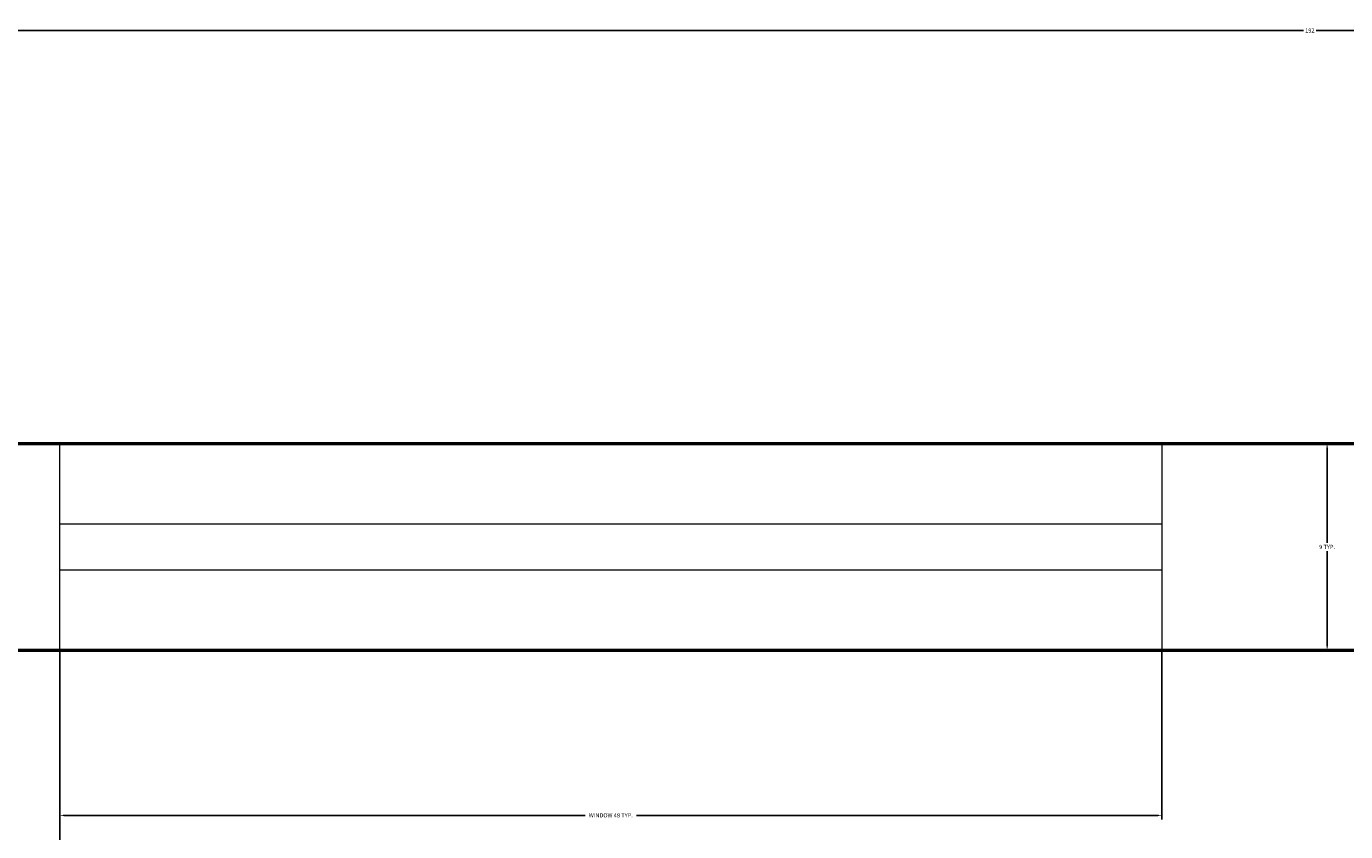
# Model space of a CAD drawing. Units: inches. Extents: x 2621 to 2849, y 2066 to 2463.
# Tile 18 of 28: x 2679 to 2736, y 2427 to 2463. Entities that reach past the tile are written whole.
import ezdxf

# ---------------------------------------------------------------- set-up
doc = ezdxf.new("R2010")
doc.units = ezdxf.units.IN
for name, color, linetype, lineweight in [('A-ANNO-DIMS', 2, 'Continuous', 18), ('A-GLAZ', 4, 'Continuous', 18), ('A-WALL', 7, 'Continuous', 50)]:
    doc.layers.add(name, color=color, linetype=linetype, lineweight=lineweight)
doc.styles.get("Standard").update_dxf_attribs({"font": 'arial.ttf'})
doc.dimstyles.get("Standard").update_dxf_attribs({"dimtxt": 0.18, "dimasz": 0.18, "dimexe": 0.18, "dimexo": 0.0625, "dimgap": 0.09, "dimtad": 0, "dimtih": 1, "dimtoh": 1, "dimdec": 4, "dimzin": 0, "dimdsep": 46, "dimtxsty": 'Standard', "dimcen": 0.09, "dimadec": 0, "dimazin": 0, "dimtfac": 1, "dimtdec": 4, "dimtofl": 0, "dimtmove": 0, "dimatfit": 3, "dimfxl": 1, "dimtolj": 1, "dimtzin": 0, "dimarcsym": 0})

# ---------------------------------------------------------------- blocks, each defined once
blk = doc.blocks.new('WIN-48IN')
for p, q in [((0, 5.5), (48, 5.5)), ((0, 3.5), (48, 3.5))]:
    blk.add_line(p, q)
for points in [[(0, 0), (0, 9)], [(48, 9), (48, 0)]]:
    blk.add_lwpolyline(points)
blk = doc.blocks.new('*D33')
at = {"layer": 'A-ANNO-DIMS', "color": 0, "lineweight": -2, "transparency": 16777216}
for p, q in [((2680.422, 2435.312), (2680.422, 2427.995)), ((2728.422, 2435.312), (2728.422, 2427.995)), ((2680.602, 2428.175), (2703.304, 2428.175)), ((2728.242, 2428.175), (2705.54, 2428.175))]:
    blk.add_line(p, q, dxfattribs=at)
at = {"layer": 'A-ANNO-DIMS', "color": 0, "transparency": 16777216}
for points in [[(2680.602, 2428.205), (2680.602, 2428.145), (2680.422, 2428.175)], [(2728.242, 2428.205), (2728.242, 2428.145), (2728.422, 2428.175)]]:
    blk.add_solid(points, dxfattribs=at)
at = {"layer": 'Defpoints', "color": 0, "transparency": 16777216}
for p in [(2680.422, 2435.375), (2728.422, 2435.375), (2728.422, 2428.175)]:
    blk.add_point(p, dxfattribs=at)
at = {"layer": 'A-ANNO-DIMS', "color": 0, "transparency": 16777216, "insert": (2704.422, 2428.175), "char_height": 0.18, "attachment_point": 5}
blk.add_mtext('\\A1;WINDOW 48 TYP.', dxfattribs=at)
blk = doc.blocks.new('*D34')
at = {"layer": 'A-ANNO-DIMS', "color": 0, "lineweight": -2, "transparency": 16777216}
for p, q in [((2728.484, 2444.375), (2735.802, 2444.375)), ((2735.622, 2444.195), (2735.622, 2440.056)), ((2735.622, 2435.555), (2735.622, 2439.693)), ((2728.484, 2435.375), (2735.802, 2435.375))]:
    blk.add_line(p, q, dxfattribs=at)
at = {"layer": 'A-ANNO-DIMS', "color": 0, "transparency": 16777216}
for points in [[(2735.592, 2444.195), (2735.652, 2444.195), (2735.622, 2444.375)], [(2735.592, 2435.555), (2735.652, 2435.555), (2735.622, 2435.375)]]:
    blk.add_solid(points, dxfattribs=at)
at = {"layer": 'Defpoints', "color": 0, "transparency": 16777216}
for p in [(2728.422, 2444.375), (2735.622, 2444.375), (2728.422, 2435.375)]:
    blk.add_point(p, dxfattribs=at)
at = {"layer": 'A-ANNO-DIMS', "color": 0, "transparency": 16777216, "insert": (2735.622, 2439.875), "char_height": 0.18, "attachment_point": 5}
blk.add_mtext('\\A1;9 TYP.', dxfattribs=at)
blk = doc.blocks.new('*D35')
at = {"layer": 'A-ANNO-DIMS', "color": 0, "lineweight": -2, "transparency": 16777216}
for p, q in [((2638.87, 2444.437), (2638.87, 2462.558)), ((2639.05, 2462.378), (2734.591, 2462.378)), ((2830.69, 2462.378), (2735.15, 2462.378)), ((2830.87, 2444.437), (2830.87, 2462.558))]:
    blk.add_line(p, q, dxfattribs=at)
at = {"layer": 'A-ANNO-DIMS', "color": 0, "transparency": 16777216}
for points in [[(2639.05, 2462.408), (2639.05, 2462.348), (2638.87, 2462.378)], [(2830.69, 2462.408), (2830.69, 2462.348), (2830.87, 2462.378)]]:
    blk.add_solid(points, dxfattribs=at)
at = {"layer": 'Defpoints', "color": 0, "transparency": 16777216}
for p in [(2830.87, 2462.378), (2638.87, 2444.375), (2830.87, 2444.375)]:
    blk.add_point(p, dxfattribs=at)
at = {"layer": 'A-ANNO-DIMS', "color": 0, "transparency": 16777216, "insert": (2734.87, 2462.378), "char_height": 0.18, "attachment_point": 5}
blk.add_mtext('\\A1;192', dxfattribs=at)
blk = doc.blocks.new('*D37')
at = {"layer": 'A-ANNO-DIMS', "color": 0, "lineweight": -2, "transparency": 16777216}
for p, q in [((2647.87, 2435.312), (2647.87, 2417.191)), ((2680.422, 2435.312), (2680.422, 2417.191)), ((2648.05, 2417.371), (2663.752, 2417.371)), ((2680.242, 2417.371), (2664.54, 2417.371))]:
    blk.add_line(p, q, dxfattribs=at)
at = {"layer": 'A-ANNO-DIMS', "color": 0, "transparency": 16777216}
for points in [[(2648.05, 2417.401), (2648.05, 2417.341), (2647.87, 2417.371)], [(2680.242, 2417.401), (2680.242, 2417.341), (2680.422, 2417.371)]]:
    blk.add_solid(points, dxfattribs=at)
at = {"layer": 'Defpoints', "color": 0, "transparency": 16777216}
for p in [(2647.87, 2435.375), (2680.422, 2435.375), (2647.87, 2417.371)]:
    blk.add_point(p, dxfattribs=at)
at = {"layer": 'A-ANNO-DIMS', "color": 0, "transparency": 16777216, "insert": (2664.146, 2417.371), "char_height": 0.18, "attachment_point": 5}
blk.add_mtext('\\A1;32.55', dxfattribs=at)
blk = doc.blocks.new('*D68')
at = {"layer": 'A-ANNO-DIMS', "color": 0, "lineweight": -2, "transparency": 16777216}
for p, q in [((2745.808, 2435.375), (2620.687, 2435.375)), ((2620.867, 2435.195), (2620.867, 2405.556)), ((2620.867, 2375.555), (2620.867, 2405.193)), ((2745.808, 2375.375), (2620.687, 2375.375))]:
    blk.add_line(p, q, dxfattribs=at)
at = {"layer": 'A-ANNO-DIMS', "color": 0, "transparency": 16777216}
for points in [[(2620.837, 2435.195), (2620.897, 2435.195), (2620.867, 2435.375)], [(2620.837, 2375.555), (2620.897, 2375.555), (2620.867, 2375.375)]]:
    blk.add_solid(points, dxfattribs=at)
at = {"layer": 'Defpoints', "color": 0, "transparency": 16777216}
for p in [(2620.867, 2435.375), (2745.87, 2435.375), (2745.87, 2375.375)]:
    blk.add_point(p, dxfattribs=at)
at = {"layer": 'A-ANNO-DIMS', "color": 0, "transparency": 16777216, "insert": (2620.867, 2405.375), "char_height": 0.18, "attachment_point": 5}
blk.add_mtext('\\A1;60', dxfattribs=at)

msp = doc.modelspace()

# ---------------------------------------------------------------- linework, layer by layer
at = {"layer": 'A-WALL'}
msp.add_line((2647.8701, 2435.3746), (2763.8701, 2435.3746), dxfattribs=at)
msp.add_lwpolyline([(2761.8701, 2084.3746), (2638.8701, 2084.3746), (2638.8701, 2444.3746), (2830.8701, 2444.3746), (2830.8701, 2084.3746), (2797.8701, 2084.3746)], dxfattribs=at)

# ---------------------------------------------------------------- block references
at = {"layer": 'A-GLAZ'}
msp.add_blockref('WIN-48IN', (2680.4219, 2435.3746), dxfattribs=at)

# ---------------------------------------------------------------- dimensions: what is measured, and where the dimension line sits
at = {"layer": 'A-ANNO-DIMS'}
dim = msp.add_linear_dim(base=(2830.8701, 2462.3781), p1=(2638.8701, 2444.3746), p2=(2830.8701, 2444.3746), dimstyle='Standard', override={"dimdec": 0, "dimlfac": 1, "dimrnd": 0, "dimzin": 0, "dimdsep": 46, "dimlunit": 2}, dxfattribs=at)
dim.commit()
dim.dimension.update_dxf_attribs({"geometry": '*D35', "text_midpoint": (2734.8701, 2462.3781)})
dim = msp.add_linear_dim(base=(2735.6219, 2444.3746), p1=(2728.4219, 2435.3746), p2=(2728.4219, 2444.3746), angle=90, text='<> TYP.', dimstyle='Standard', override={"dimdec": 0, "dimlfac": 1, "dimrnd": 0, "dimzin": 0, "dimdsep": 46, "dimlunit": 2}, dxfattribs=at)
dim.commit()
dim.dimension.update_dxf_attribs({"geometry": '*D34', "text_midpoint": (2735.6219, 2439.8746)})
for base, p1, p2, angle, override, picture, middle in [((2620.8666, 2435.3746), (2745.8701, 2375.3746), (2745.8701, 2435.3746), 90, {"dimdec": 0, "dimlfac": 1, "dimrnd": 0, "dimzin": 0, "dimdsep": 46, "dimlunit": 2}, '*D68', (2620.8666, 2405.3746)), ((2647.8701, 2417.3711), (2680.4219, 2435.3746), (2647.8701, 2435.3746), 180, {"dimdec": 2, "dimlfac": 1, "dimrnd": 0, "dimzin": 0, "dimdsep": 46, "dimlunit": 2}, '*D37', (2664.146, 2417.3711))]:
    dim = msp.add_linear_dim(base=base, p1=p1, p2=p2, angle=angle, dimstyle='Standard', override=override, dxfattribs=at)
    dim.commit()
    dim.dimension.update_dxf_attribs({"geometry": picture, "text_midpoint": middle})
dim = msp.add_linear_dim(base=(2728.4219, 2428.1746), p1=(2680.4219, 2435.3746), p2=(2728.4219, 2435.3746), text='WINDOW <> TYP.', dimstyle='Standard', override={"dimdec": 0, "dimlfac": 1, "dimrnd": 0, "dimzin": 0, "dimdsep": 46, "dimlunit": 2}, dxfattribs=at)
dim.commit()
dim.dimension.update_dxf_attribs({"geometry": '*D33', "text_midpoint": (2704.4219, 2428.1746)})

doc.saveas('drawing.dxf')
